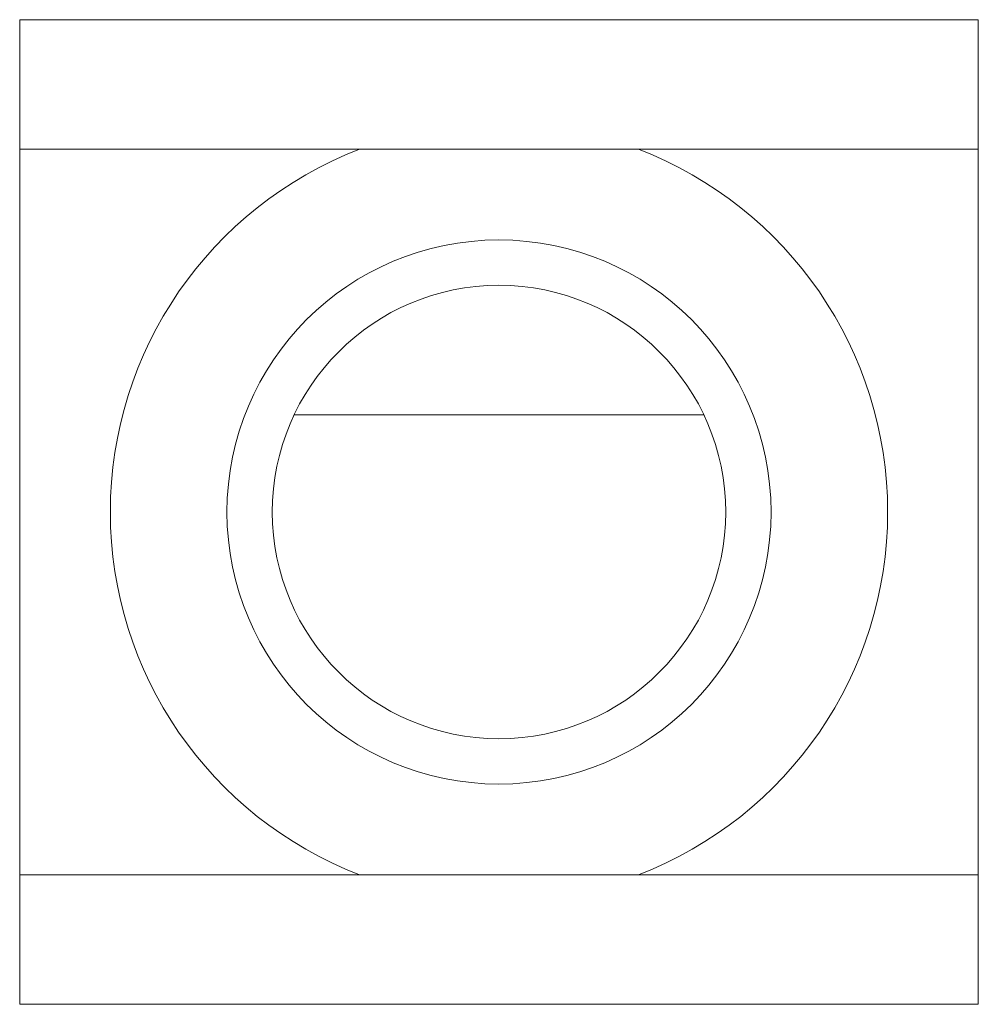
# Model space of a CAD drawing. Units: millimetres. Extents: x 2523.7 to 2597.7, y 1594.7 to 1670.7.
import ezdxf

# ---------------------------------------------------------------- set-up
doc = ezdxf.new("R2010")
doc.units = ezdxf.units.MM
doc.layers.add('M-CONS', color=8, linetype='Continuous', lineweight=18)

msp = doc.modelspace()

# ---------------------------------------------------------------- linework, layer by layer
at = {"layer": 'M-CONS'}
for p, q in [((2523.713, 1670.658), (2523.713, 1660.658)), ((2523.713, 1660.658), (2597.713, 1660.658)), ((2560.713, 1640.158, 155), (2544.902, 1640.158, 155)), ((2544.902, 1640.158, 155), (2576.525, 1640.158, 155))]:
    msp.add_line(p, q, dxfattribs=at)
at = {"layer": 'M-CONS', "extrusion": (0, 1, 0)}
for p, q in [((2523.713, 1604.658, -10), (2547.81, 1604.658, -50.649)), ((2597.713, 1604.658, -10), (2573.616, 1604.658, -50.649))]:
    msp.add_line(p, q, dxfattribs=at)
at = {"layer": 'M-CONS'}
msp.add_lwpolyline([(2523.713, 1670.658), (2523.713, 1594.658), (2597.713, 1594.658), (2597.713, 1670.658)], close=True, dxfattribs=at)
msp.add_lwpolyline([(2523.713, 1594.658), (2523.713, 1604.658), (2597.713, 1604.658)], dxfattribs=at)
for radius in [21, 17.5]:
    msp.add_circle((2560.713, 1632.658), radius, dxfattribs=at)
at = {"layer": 'M-CONS', "extrusion": (0, -1, 0)}
for centre, radius in [((2560.713, -43, -1604.658), 15), ((2560.713, -43, -1604.658), 5), ((2560.713, -43, -1594.658), 15), ((2560.713, -43, -1594.658), 5)]:
    msp.add_circle(centre, radius, dxfattribs=at)
at = {"layer": 'M-CONS'}
for start, end in [(111.03947, 248.96053), (291.03947, 68.96053)]:
    msp.add_arc((2560.713, 1632.658), 30, start, end, dxfattribs=at)

doc.saveas('drawing.dxf')
